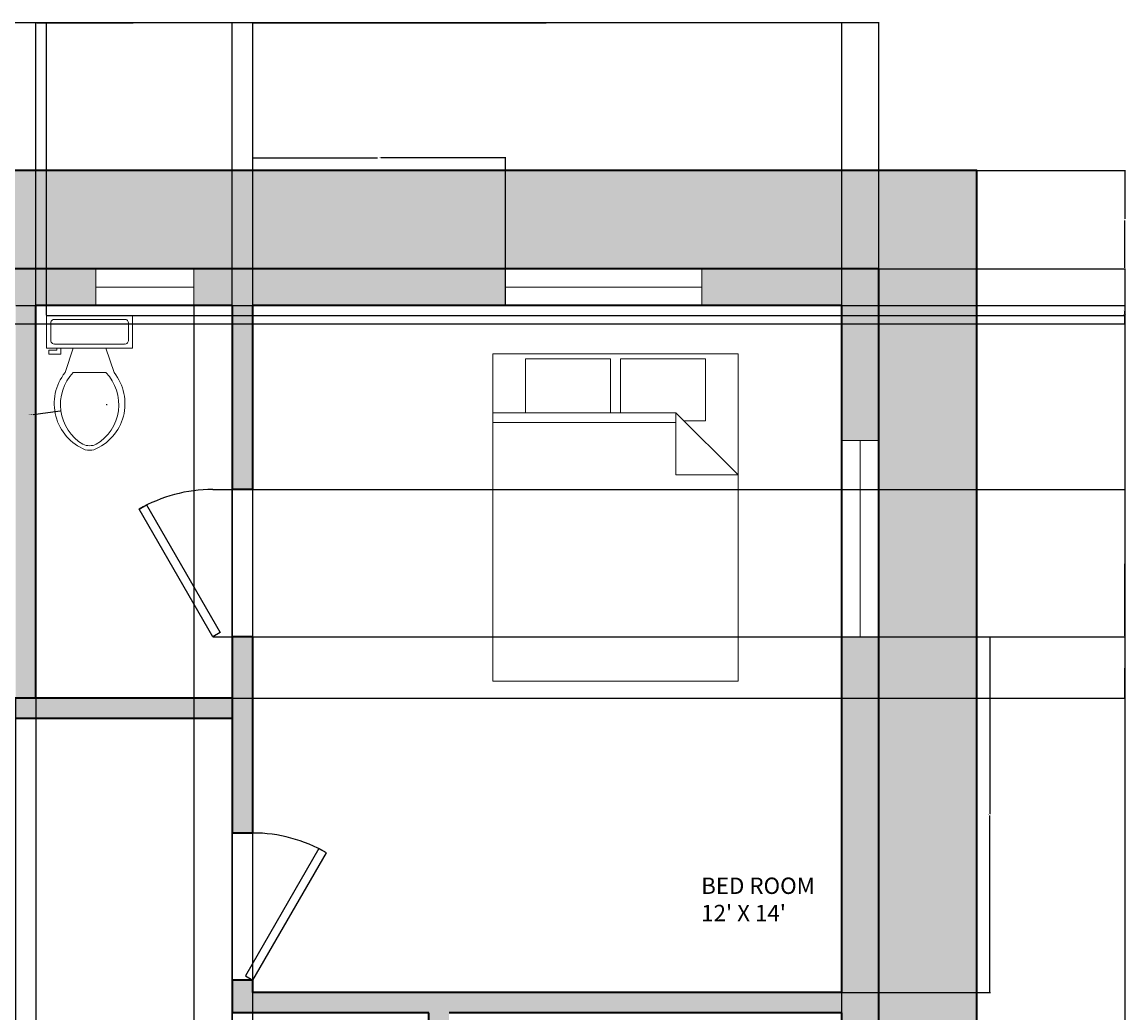
# Model space of a CAD drawing. Units: inches. Extents: x -7 to 546, y -27 to 766.
# Tile 9 of 9: x 276 to 546, y 524 to 766. Entities that reach past the tile are written whole.
import ezdxf

# ---------------------------------------------------------------- set-up
doc = ezdxf.new("R2010")
doc.units = ezdxf.units.IN
doc.header["$MEASUREMENT"] = 0
for name, color, linetype, lineweight in [('A-ANNO-DIMS', 2, 'Continuous', 18), ('A-AREA-IDEN', 7, 'Continuous', 18), ('A-FLOR-FIXT', 9, 'Continuous', 18), ('A-WALL', 7, 'Continuous', 35), ('C-PROP', 7, 'Continuous', 35), ('doors', 40, 'Continuous', 25), ('furniture', 220, 'Continuous', 18), ('window', 30, 'Continuous', 20)]:
    doc.layers.add(name, color=color, linetype=linetype, lineweight=lineweight)
doc.layers.add('A-WALL-PATT', color=251, linetype='Continuous', lineweight=13, true_color=0x636466)
doc.layers.add('L-PLNT-PATT', color=85, linetype='Continuous', lineweight=13, true_color=0x58ba48)
doc.styles.get("Standard").update_dxf_attribs({"font": 'arial.ttf'})
doc.dimstyles.get("Standard").update_dxf_attribs({"dimtxt": 0.18, "dimasz": 0.18, "dimexe": 0.18, "dimexo": 0.0625, "dimgap": 0.09, "dimtad": 0, "dimtih": 1, "dimtoh": 1, "dimdec": 4, "dimzin": 0, "dimdsep": 46, "dimtxsty": 'Standard', "dimcen": 0.09, "dimadec": 0, "dimazin": 0, "dimtfac": 1, "dimtdec": 4, "dimtofl": 0, "dimtmove": 0, "dimatfit": 3, "dimfxl": 1, "dimtolj": 1, "dimtzin": 0, "dimarcsym": 0})

# ---------------------------------------------------------------- blocks, each defined once
blk = doc.blocks.new('*U11')
for p, q in [((0, 0), (0, 100)), ((750, 0), (750, 100))]:
    blk.add_line(p, q)
blk.add_lwpolyline([(0, 0), (649.5, -375), (671.4, -337.1), (21.9, 37.9)], close=True)
blk.add_arc((0, 0), 750, 330, 0)
blk = doc.blocks.new('*U10')
for p, q in [((0, 0), (0, -100)), ((750, 0), (750, -100))]:
    blk.add_line(p, q)
blk.add_lwpolyline([(0, 0), (649.5, 375), (671.4, 337.1), (21.9, -37.9)], close=True)
blk.add_arc((0, 0), 750, 0, 30)
blk = doc.blocks.new('Bed - Queen')
for p, q in [((0, -80.00003), (0, 0)), ((0, 0), (59.99999, 0)), ((59.99999, 0), (59.99999, -80.00003)), ((7.99999, -1.2), (28.79998, -1.2)), ((7.99999, -14.4), (7.99999, -1.2)), ((28.79998, -1.2), (28.79998, -14.4)), ((31.19999, -1.2), (51.99999, -1.2)), ((31.19999, -14.4), (31.19999, -1.2)), ((51.99999, -1.2), (51.99999, -16.4)), ((0, -14.4), (44.8, -14.4)), ((59.99999, -29.6), (44.8, -14.4)), ((44.8, -14.4), (44.8, -29.6)), ((44.8, -16.8), (0, -16.8)), ((51.99999, -16.4), (46.79936, -16.4)), ((44.8, -29.6), (59.99999, -29.6)), ((59.99999, -80.00003), (0, -80.00003))]:
    blk.add_line(p, q)
blk = doc.blocks.new('Toilet - top')
for p, q in [((9.5, -6), (9.5, -2)), ((-8, -8.5), (-8, -8)), ((-7, -8), (-7, -9.5)), ((-4, -8), (-6, -14)), ((4, -8), (6, -14)), ((-10, -8.5), (-8, -8.5)), ((-10, -9.5), (-10, -8.5)), ((-7, -9.5), (-10, -9.5)), ((4, -14), (-4, -14))]:
    blk.add_line(p, q)
blk.add_lwpolyline([(10.5, -8), (10.5, 0), (-10.5, 0), (-10.5, -8)], close=True)
for points in [[(-9.5, -2), (-9.5, -6)], [(8.5, -1), (-8.5, -1)], [(-8.5, -7), (8.5, -7)]]:
    blk.add_lwpolyline(points)
for centre, radius, start, end in [((-8.62, -1.88), 0.884, 81.8699, 188.1301), ((8.62, -1.88), 0.884, 351.8699, 98.1301), ((-8.62, -6.12), 0.884, 171.8699, 278.1301), ((8.62, -6.12), 0.884, 261.8699, 8.1301), ((3.52, -21.58), 12.17, 141.4691, 247.9714), ((4.2, -21.82), 11.33, 136.3677, 238.9468), ((-3.52, -21.58), 12.17, 292.0284, 38.5307), ((-4.2, -21.82), 11.33, 301.053, 43.6321), ((0, -27.88), 4, 245.7318, 294.2682), ((0, -29), 4, 254.8605, 285.1395)]:
    blk.add_arc(centre, radius, start, end)
blk = doc.blocks.new('WIN-48IN')
for p, q in [((0, 9), (0, 0)), ((48, 9), (0, 9)), ((0, 9), (0, 4.5)), ((48, 0), (48, 9)), ((0, 4.5), (48, 4.5)), ((0, 0), (48, 0))]:
    blk.add_line(p, q)
blk = doc.blocks.new('WIN-24IN')
for p, q in [((0, 9), (0, 0)), ((24, 9), (0, 9)), ((0, 9), (0, 4.5)), ((24, 0), (24, 9)), ((0, 4.5), (24, 4.5)), ((0, 0), (24, 0))]:
    blk.add_line(p, q)
blk = doc.blocks.new('*D32')
at = {"layer": 'A-ANNO-DIMS', "color": 0, "lineweight": -2, "transparency": 16777216}
for p, q in [((53.23, 705.81), (53.23, 766.05)), ((53.41, 765.87), (268.94, 765.87)), ((485.05, 765.87), (269.52, 765.87)), ((485.23, 705.81), (485.23, 766.05))]:
    blk.add_line(p, q, dxfattribs=at)
at = {"layer": 'A-ANNO-DIMS', "color": 0, "transparency": 16777216}
for points in [[(53.41, 765.9), (53.41, 765.84), (53.23, 765.87)], [(485.05, 765.9), (485.05, 765.84), (485.23, 765.87)]]:
    blk.add_solid(points, dxfattribs=at)
at = {"layer": 'Defpoints', "color": 0, "transparency": 16777216}
for p in [(485.23, 765.87), (53.23, 705.74), (485.23, 705.74)]:
    blk.add_point(p, dxfattribs=at)
at = {"layer": 'A-ANNO-DIMS', "color": 0, "transparency": 16777216, "insert": (269.23, 765.87), "char_height": 0.18, "attachment_point": 5}
blk.add_mtext('\\A1;432', dxfattribs=at)
blk = doc.blocks.new('*D33')
at = {"layer": 'A-ANNO-DIMS', "color": 0, "lineweight": -2, "transparency": 16777216}
for p, q in [((485.29, 705.74), (545.54, 705.74)), ((545.36, 705.56), (545.36, 357.93)), ((545.36, 9.92), (545.36, 357.56)), ((461.29, 9.74), (545.54, 9.74))]:
    blk.add_line(p, q, dxfattribs=at)
at = {"layer": 'A-ANNO-DIMS', "color": 0, "transparency": 16777216}
for points in [[(545.33, 705.56), (545.39, 705.56), (545.36, 705.74)], [(545.33, 9.92), (545.39, 9.92), (545.36, 9.74)]]:
    blk.add_solid(points, dxfattribs=at)
at = {"layer": 'Defpoints', "color": 0, "transparency": 16777216}
for p in [(485.23, 705.74), (461.23, 9.74), (545.36, 9.74)]:
    blk.add_point(p, dxfattribs=at)
at = {"layer": 'A-ANNO-DIMS', "color": 0, "transparency": 16777216, "insert": (545.36, 357.74), "char_height": 0.18, "attachment_point": 5}
blk.add_mtext('\\A1;696', dxfattribs=at)
blk = doc.blocks.new('*D35')
at = {"layer": 'A-ANNO-DIMS', "color": 0, "lineweight": -2, "transparency": 16777216}
for p, q in [((509.29, 729.74), (545.54, 729.74)), ((545.36, 729.56), (545.36, 717.92)), ((545.36, 705.92), (545.36, 717.56)), ((485.29, 705.74), (545.54, 705.74))]:
    blk.add_line(p, q, dxfattribs=at)
at = {"layer": 'A-ANNO-DIMS', "color": 0, "transparency": 16777216}
for points in [[(545.33, 729.56), (545.39, 729.56), (545.36, 729.74)], [(545.33, 705.92), (545.39, 705.92), (545.36, 705.74)]]:
    blk.add_solid(points, dxfattribs=at)
at = {"layer": 'Defpoints', "color": 0, "transparency": 16777216}
for p in [(509.23, 729.74), (485.23, 705.74), (545.36, 705.74)]:
    blk.add_point(p, dxfattribs=at)
at = {"layer": 'A-ANNO-DIMS', "color": 0, "transparency": 16777216, "insert": (545.36, 717.74), "char_height": 0.18, "attachment_point": 5}
blk.add_mtext('\\A1;24', dxfattribs=at)
blk = doc.blocks.new('*D37')
at = {"layer": 'A-ANNO-DIMS', "color": 0, "lineweight": -2, "transparency": 16777216}
for p, q in [((279.23, 696.81), (279.23, 766.05)), ((279.41, 765.87), (303.01, 765.87)), ((327.05, 765.87), (303.45, 765.87)), ((327.23, 696.81), (327.23, 766.05))]:
    blk.add_line(p, q, dxfattribs=at)
at = {"layer": 'A-ANNO-DIMS', "color": 0, "transparency": 16777216}
for points in [[(279.41, 765.9), (279.41, 765.84), (279.23, 765.87)], [(327.05, 765.9), (327.05, 765.84), (327.23, 765.87)]]:
    blk.add_solid(points, dxfattribs=at)
at = {"layer": 'Defpoints', "color": 0, "transparency": 16777216}
for p in [(327.23, 765.87), (279.23, 696.74), (327.23, 696.74)]:
    blk.add_point(p, dxfattribs=at)
at = {"layer": 'A-ANNO-DIMS', "color": 0, "transparency": 16777216, "insert": (303.23, 765.87), "char_height": 0.18, "attachment_point": 5}
blk.add_mtext('\\A1;48', dxfattribs=at)
blk = doc.blocks.new('*D40')
at = {"layer": 'A-ANNO-DIMS', "color": 0, "lineweight": -2, "transparency": 16777216}
for p, q in [((327.29, 651.74), (545.54, 651.74)), ((545.36, 651.56), (545.36, 633.93)), ((545.36, 615.92), (545.36, 633.56)), ((327.29, 615.74), (545.54, 615.74))]:
    blk.add_line(p, q, dxfattribs=at)
at = {"layer": 'A-ANNO-DIMS', "color": 0, "transparency": 16777216}
for points in [[(545.33, 651.56), (545.39, 651.56), (545.36, 651.74)], [(545.33, 615.92), (545.39, 615.92), (545.36, 615.74)]]:
    blk.add_solid(points, dxfattribs=at)
at = {"layer": 'Defpoints', "color": 0, "transparency": 16777216}
for p in [(327.23, 651.74), (545.36, 651.74), (327.23, 615.74)]:
    blk.add_point(p, dxfattribs=at)
at = {"layer": 'A-ANNO-DIMS', "color": 0, "transparency": 16777216, "insert": (545.36, 633.74), "char_height": 0.18, "attachment_point": 5}
blk.add_mtext('\\A1;36', dxfattribs=at)
blk = doc.blocks.new('*D41')
at = {"layer": 'A-ANNO-DIMS', "color": 0, "lineweight": -2, "transparency": 16777216}
for p, q in [((274.23, 600.68), (274.23, -26.56)), ((279.23, 600.68), (279.23, -26.56)), ((274.41, -26.38), (276.58, -26.38)), ((279.05, -26.38), (276.88, -26.38))]:
    blk.add_line(p, q, dxfattribs=at)
at = {"layer": 'A-ANNO-DIMS', "color": 0, "transparency": 16777216}
for points in [[(274.41, -26.35), (274.41, -26.41), (274.23, -26.38)], [(279.05, -26.35), (279.05, -26.41), (279.23, -26.38)]]:
    blk.add_solid(points, dxfattribs=at)
at = {"layer": 'Defpoints', "color": 0, "transparency": 16777216}
for p in [(274.23, 600.74), (279.23, 600.74), (279.23, -26.38)]:
    blk.add_point(p, dxfattribs=at)
at = {"layer": 'A-ANNO-DIMS', "color": 0, "transparency": 16777216, "insert": (276.73, -26.38), "char_height": 0.18, "attachment_point": 5}
blk.add_mtext('\\A1;5', dxfattribs=at)
blk = doc.blocks.new('*D43')
at = {"layer": 'A-ANNO-DIMS', "color": 0, "lineweight": -2, "transparency": 16777216}
for p, q in [((317.84, 696.68), (317.84, -26.56)), ((327.23, 696.68), (327.23, -26.56)), ((318.02, -26.38), (322.21, -26.38)), ((327.05, -26.38), (322.86, -26.38))]:
    blk.add_line(p, q, dxfattribs=at)
at = {"layer": 'A-ANNO-DIMS', "color": 0, "transparency": 16777216}
for points in [[(318.02, -26.35), (318.02, -26.41), (317.84, -26.38)], [(327.05, -26.35), (327.05, -26.41), (327.23, -26.38)]]:
    blk.add_solid(points, dxfattribs=at)
at = {"layer": 'Defpoints', "color": 0, "transparency": 16777216}
for p in [(317.84, 696.74), (327.23, 696.74), (327.23, -26.38)]:
    blk.add_point(p, dxfattribs=at)
at = {"layer": 'A-ANNO-DIMS', "color": 0, "transparency": 16777216, "insert": (322.54, -26.38), "char_height": 0.18, "attachment_point": 5}
blk.add_mtext('\\A1;9.39', dxfattribs=at)
blk = doc.blocks.new('*D44')
at = {"layer": 'A-ANNO-DIMS', "color": 0, "lineweight": -2, "transparency": 16777216}
for p, q in [((327.29, 615.74), (545.54, 615.74)), ((545.36, 615.56), (545.36, 608.43)), ((545.36, 600.92), (545.36, 608.06)), ((327.29, 600.74), (545.54, 600.74))]:
    blk.add_line(p, q, dxfattribs=at)
at = {"layer": 'A-ANNO-DIMS', "color": 0, "transparency": 16777216}
for points in [[(545.33, 615.56), (545.39, 615.56), (545.36, 615.74)], [(545.33, 600.92), (545.39, 600.92), (545.36, 600.74)]]:
    blk.add_solid(points, dxfattribs=at)
at = {"layer": 'Defpoints', "color": 0, "transparency": 16777216}
for p in [(327.23, 615.74), (545.36, 615.74), (327.23, 600.74)]:
    blk.add_point(p, dxfattribs=at)
at = {"layer": 'A-ANNO-DIMS', "color": 0, "transparency": 16777216, "insert": (545.36, 608.24), "char_height": 0.18, "attachment_point": 5}
blk.add_mtext('\\A1;15', dxfattribs=at)
blk = doc.blocks.new('*D57')
at = {"layer": 'A-ANNO-DIMS', "color": 0, "lineweight": -2, "transparency": 16777216}
for p, q in [((332.23, 273.81), (332.23, 766.05)), ((332.41, 765.87), (403.95, 765.87)), ((476.05, 765.87), (404.51, 765.87)), ((476.23, 273.81), (476.23, 766.05))]:
    blk.add_line(p, q, dxfattribs=at)
at = {"layer": 'A-ANNO-DIMS', "color": 0, "transparency": 16777216}
for points in [[(332.41, 765.9), (332.41, 765.84), (332.23, 765.87)], [(476.05, 765.9), (476.05, 765.84), (476.23, 765.87)]]:
    blk.add_solid(points, dxfattribs=at)
at = {"layer": 'Defpoints', "color": 0, "transparency": 16777216}
for p in [(476.23, 765.87), (332.23, 273.74), (476.23, 273.74)]:
    blk.add_point(p, dxfattribs=at)
at = {"layer": 'A-ANNO-DIMS', "color": 0, "transparency": 16777216, "insert": (404.23, 765.87), "char_height": 0.18, "attachment_point": 5}
blk.add_mtext('\\A1;144', dxfattribs=at)
blk = doc.blocks.new('*D70')
at = {"layer": 'A-ANNO-DIMS', "color": 0, "lineweight": -2, "transparency": 16777216}
for p, q in [((332.23, 696.81), (332.23, 733.05)), ((332.41, 732.87), (362.71, 732.87)), ((393.79, 732.87), (363.5, 732.87)), ((393.97, 696.81), (393.97, 733.05))]:
    blk.add_line(p, q, dxfattribs=at)
at = {"layer": 'A-ANNO-DIMS', "color": 0, "transparency": 16777216}
for points in [[(332.41, 732.9), (332.41, 732.84), (332.23, 732.87)], [(393.79, 732.9), (393.79, 732.84), (393.97, 732.87)]]:
    blk.add_solid(points, dxfattribs=at)
at = {"layer": 'Defpoints', "color": 0, "transparency": 16777216}
for p in [(393.97, 732.87), (332.23, 696.74), (393.97, 696.74)]:
    blk.add_point(p, dxfattribs=at)
at = {"layer": 'A-ANNO-DIMS', "color": 0, "transparency": 16777216, "insert": (363.1, 732.87), "char_height": 0.18, "attachment_point": 5}
blk.add_mtext('\\A1;61.74', dxfattribs=at)
blk = doc.blocks.new('*D75')
at = {"layer": 'A-ANNO-DIMS', "color": 0, "lineweight": -2, "transparency": 16777216}
for p, q in [((476.29, 615.69), (512.54, 615.69)), ((512.36, 615.51), (512.36, 572.4)), ((512.36, 528.92), (512.36, 572.03)), ((476.29, 528.74), (512.54, 528.74))]:
    blk.add_line(p, q, dxfattribs=at)
at = {"layer": 'A-ANNO-DIMS', "color": 0, "transparency": 16777216}
for points in [[(512.33, 615.51), (512.39, 615.51), (512.36, 615.69)], [(512.33, 528.92), (512.39, 528.92), (512.36, 528.74)]]:
    blk.add_solid(points, dxfattribs=at)
at = {"layer": 'Defpoints', "color": 0, "transparency": 16777216}
for p in [(476.23, 615.69), (476.23, 528.74), (512.36, 528.74)]:
    blk.add_point(p, dxfattribs=at)
at = {"layer": 'A-ANNO-DIMS', "color": 0, "transparency": 16777216, "insert": (512.36, 572.22), "char_height": 0.18, "attachment_point": 5}
blk.add_mtext('\\A1;86.95', dxfattribs=at)
blk = doc.blocks.new('*D81')
at = {"layer": 'A-ANNO-DIMS', "color": 0, "lineweight": -2, "transparency": 16777216}
for p, q in [((62.23, 240.81), (62.23, 766.05)), ((62.41, 765.87), (194.44, 765.87)), ((327.05, 765.87), (195.02, 765.87)), ((327.23, 234.81), (327.23, 766.05))]:
    blk.add_line(p, q, dxfattribs=at)
at = {"layer": 'A-ANNO-DIMS', "color": 0, "transparency": 16777216}
for points in [[(62.41, 765.9), (62.41, 765.84), (62.23, 765.87)], [(327.05, 765.9), (327.05, 765.84), (327.23, 765.87)]]:
    blk.add_solid(points, dxfattribs=at)
at = {"layer": 'Defpoints', "color": 0, "transparency": 16777216}
for p in [(327.23, 765.87), (62.23, 240.74), (327.23, 234.74)]:
    blk.add_point(p, dxfattribs=at)
at = {"layer": 'A-ANNO-DIMS', "color": 0, "transparency": 16777216, "insert": (194.73, 765.87), "char_height": 0.18, "attachment_point": 5}
blk.add_mtext('\\A1;265', dxfattribs=at)
blk = doc.blocks.new('*D86')
at = {"layer": 'A-ANNO-DIMS', "color": 0, "lineweight": -2, "transparency": 16777216}
for p, q in [((274.29, 696.74), (545.54, 696.74)), ((545.36, 696.56), (545.36, 694.67)), ((545.36, 692.41), (545.36, 694.31)), ((268.8, 692.23), (545.54, 692.23))]:
    blk.add_line(p, q, dxfattribs=at)
at = {"layer": 'A-ANNO-DIMS', "color": 0, "transparency": 16777216}
for points in [[(545.33, 696.56), (545.39, 696.56), (545.36, 696.74)], [(545.33, 692.41), (545.39, 692.41), (545.36, 692.23)]]:
    blk.add_solid(points, dxfattribs=at)
at = {"layer": 'Defpoints', "color": 0, "transparency": 16777216}
for p in [(274.23, 696.74), (268.74, 692.23), (545.36, 692.23)]:
    blk.add_point(p, dxfattribs=at)
at = {"layer": 'A-ANNO-DIMS', "color": 0, "transparency": 16777216, "insert": (545.36, 694.49), "char_height": 0.18, "attachment_point": 5}
blk.add_mtext('\\A1;4.512', dxfattribs=at)
blk = doc.blocks.new('*D87')
at = {"layer": 'A-ANNO-DIMS', "color": 0, "lineweight": -2, "transparency": 16777216}
for p, q in [((279.23, 696.81), (279.23, 766.05)), ((279.41, 765.87), (280.14, 765.87)), ((281.66, 765.87), (280.93, 765.87)), ((281.84, 694.39), (281.84, 766.05))]:
    blk.add_line(p, q, dxfattribs=at)
at = {"layer": 'A-ANNO-DIMS', "color": 0, "transparency": 16777216}
for points in [[(279.41, 765.9), (279.41, 765.84), (279.23, 765.87)], [(281.66, 765.9), (281.66, 765.84), (281.84, 765.87)]]:
    blk.add_solid(points, dxfattribs=at)
at = {"layer": 'Defpoints', "color": 0, "transparency": 16777216}
for p in [(281.84, 765.87), (279.23, 696.74), (281.84, 694.32)]:
    blk.add_point(p, dxfattribs=at)
at = {"layer": 'A-ANNO-DIMS', "color": 0, "transparency": 16777216, "insert": (280.54, 765.87), "char_height": 0.18, "attachment_point": 5}
blk.add_mtext('\\A1;2.608', dxfattribs=at)
blk = doc.blocks.new('*D88')
at = {"layer": 'A-ANNO-DIMS', "color": 0, "lineweight": -2, "transparency": 16777216}
for p, q in [((279.29, 696.74), (545.54, 696.74)), ((545.36, 696.56), (545.36, 695.71)), ((281.9, 694.32), (545.54, 694.32)), ((545.36, 694.5), (545.36, 695.35))]:
    blk.add_line(p, q, dxfattribs=at)
at = {"layer": 'A-ANNO-DIMS', "color": 0, "transparency": 16777216}
for points in [[(545.33, 696.56), (545.39, 696.56), (545.36, 696.74)], [(545.33, 694.5), (545.39, 694.5), (545.36, 694.32)]]:
    blk.add_solid(points, dxfattribs=at)
at = {"layer": 'Defpoints', "color": 0, "transparency": 16777216}
for p in [(279.23, 696.74), (281.84, 694.32), (545.36, 694.32)]:
    blk.add_point(p, dxfattribs=at)
at = {"layer": 'A-ANNO-DIMS', "color": 0, "transparency": 16777216, "insert": (545.36, 695.53), "char_height": 0.18, "attachment_point": 5}
blk.add_mtext('\\A1;2.42', dxfattribs=at)
blk = doc.blocks.new('*D94')
at = {"layer": 'A-ANNO-DIMS', "color": 0, "lineweight": -2, "transparency": 16777216}
for p, q in [((296.45, 672.51), (296.63, 672.51)), ((296.54, 672.42), (296.54, 672.6)), ((278.57, 670.09), (285.13, 670.97))]:
    blk.add_line(p, q, dxfattribs=at)
at = {"layer": 'A-ANNO-DIMS', "color": 0, "transparency": 16777216}
blk.add_solid([(285.13, 671), (285.14, 670.94), (285.31, 671)], dxfattribs=at)
at = {"layer": 'Defpoints', "color": 0, "transparency": 16777216}
for p in [(296.54, 672.51), (285.31, 671)]:
    blk.add_point(p, dxfattribs=at)
at = {"layer": 'A-ANNO-DIMS', "color": 0, "transparency": 16777216, "insert": (277.9, 670.09), "char_height": 0.18, "attachment_point": 5}
blk.add_mtext('\\A1;6X R11.33', dxfattribs=at)

msp = doc.modelspace()

# ---------------------------------------------------------------- hatches: boundary and pattern name
at = {"layer": 'A-WALL-PATT'}
h = msp.add_hatch(color=256, dxfattribs=at)
h.dxf.hatch_style = 1
h.paths.add_polyline_path([(62.2319, 696.744), (86.6896, 696.744), (86.6896, 705.744), (53.2319, 705.744), (53.2319, 627.8642), (57.7271, 627.8642), (62.2319, 627.8642)])
h.paths.add_polyline_path([(229.7414, 705.744), (134.6896, 705.744), (134.6896, 696.744), (206.2319, 696.744), (206.2319, 567.744), (211.2319, 567.744), (211.2319, 595.744), (214.2319, 595.744), (214.2319, 600.744), (211.2319, 600.744), (211.2319, 696.744), (229.7414, 696.744)])
h.paths.add_polyline_path([(293.8423, 705.744), (253.7414, 705.744), (253.7414, 696.744), (274.2319, 696.744), (274.2319, 600.744), (279.2319, 600.744), (279.2319, 696.744), (293.8423, 696.744)])
h.paths.add_polyline_path([(393.9743, 705.744), (317.8423, 705.744), (317.8423, 696.744), (327.2319, 696.744), (327.2319, 651.744), (332.2319, 651.744), (332.2319, 696.744), (393.9743, 696.744)])
h.paths.add_polyline_path([(485.2319, 705.744), (441.9743, 705.744), (441.9743, 696.744), (476.2319, 696.744), (476.2319, 663.6898), (480.7319, 663.6898), (485.2319, 663.6898)])
h.paths.add_polyline_path([(485.2319, 615.6898), (476.2319, 615.6898), (476.2319, 528.744), (332.2319, 528.744), (332.2319, 531.744), (327.2319, 531.744), (327.2319, 523.744), (375.2319, 523.744), (375.2319, 427.744), (327.2319, 427.744), (327.2319, 419.744), (332.2319, 419.744), (332.2319, 422.744), (413.089, 422.744), (413.089, 427.744), (380.2319, 427.744), (380.2319, 523.744), (476.2319, 523.744), (476.2319, 490.9334), (485.2319, 490.9334)])
h.paths.add_polyline_path([(485.2319, 466.9334), (476.2319, 466.9334), (476.2319, 370.0932), (480.7319, 370.0932), (485.2319, 370.0932)])
h.paths.add_polyline_path([(485.2319, 322.0932), (476.2319, 322.0932), (476.2319, 278.744), (332.2319, 278.744), (332.2319, 383.744), (327.2319, 383.744), (327.2319, 273.744), (327.2319, 270.744), (332.2319, 270.744), (332.2319, 273.744), (476.2319, 273.744), (476.2319, 201.0338), (480.7319, 201.0338), (485.2319, 201.0338)])
h.paths.add_polyline_path([(485.2319, 153.0338), (476.2319, 153.0338), (476.2319, 42.744), (461.2319, 42.744), (461.2319, 33.744), (485.2319, 33.744)])
h.paths.add_polyline_path([(332.2319, 234.744), (327.2319, 234.744), (327.2319, 160.744), (315.2319, 160.744), (315.2319, 151.744), (327.2319, 151.744), (327.2319, 33.744), (332.2319, 33.744)])
h.paths.add_polyline_path([(252.2319, 151.744), (258.4464, 151.744), (264.2319, 151.744), (264.2319, 160.744), (252.2319, 160.744), (252.2319, 172.744), (247.2319, 172.744), (247.2319, 91.744), (127.2319, 91.744), (127.2319, 196.744), (122.2319, 196.744), (122.2319, 91.744), (62.2319, 91.744), (62.2319, 126.1124), (53.2319, 126.1124), (53.2319, 9.744), (62.2319, 9.744), (62.2319, 86.744), (247.2319, 86.744), (247.2319, 33.744), (252.2319, 33.744), (252.2319, 53.744)])
h.paths.add_polyline_path([(62.2319, 235.744), (122.2319, 235.744), (122.2319, 232.744), (127.2319, 232.744), (127.2319, 235.744), (247.2319, 235.744), (247.2319, 220.744), (252.2319, 220.744), (252.2319, 240.744), (250.6678, 240.744), (247.2319, 240.744), (62.2319, 240.744), (62.2319, 322.0932), (53.2319, 322.0932), (53.2319, 174.1124), (57.7271, 174.1124), (62.2319, 174.1124)])
h = msp.add_hatch(color=256, dxfattribs=at)
h.dxf.hatch_style = 1
h.paths.add_polyline_path([(327.2319, 600.744), (252.2319, 600.744), (252.2319, 595.744), (327.2319, 595.744)])
h.paths.add_polyline_path([(332.2319, 615.744), (327.2319, 615.744), (327.2319, 567.744), (332.2319, 567.744)])
h.paths.add_polyline_path([(252.2319, 600.744), (250.2319, 600.744), (250.2319, 595.744), (252.2319, 595.744)])
at = {"layer": 'L-PLNT-PATT'}
h = msp.add_hatch(color=256, dxfattribs=at)
h.dxf.hatch_style = 1
h.paths.add_polyline_path([(509.2319, 729.744), (29.2319, 729.744), (29.2319, 9.744), (53.2319, 9.744), (53.2319, 705.744), (485.2319, 705.744), (485.2319, 33.744), (461.2319, 33.744), (461.2319, 9.744), (509.2319, 9.744)])

# ---------------------------------------------------------------- linework, layer by layer
at = {"layer": 'A-WALL'}
for p, q in [((279.2319, 600.744), (279.2319, 696.744)), ((327.2319, 696.744), (279.2319, 696.744)), ((327.2319, 651.744), (327.2319, 696.744)), ((327.2319, 651.744), (327.2319, 696.744)), ((332.2319, 651.744), (332.2319, 696.744)), ((332.2319, 651.744), (332.2319, 696.744)), ((476.2319, 696.744), (332.2319, 696.744)), ((476.2319, 528.744), (476.2319, 696.744)), ((332.2319, 651.744), (327.2319, 651.744)), ((327.2319, 567.744), (327.2319, 615.744)), ((327.2319, 600.744), (327.2319, 615.744)), ((332.2319, 615.744), (327.2319, 615.744)), ((332.2319, 567.744), (332.2319, 615.744)), ((332.2319, 567.744), (332.2319, 615.744)), ((332.2319, 600.744), (332.2319, 615.744)), ((327.2319, 600.744), (250.2319, 600.744)), ((327.2319, 595.744), (250.2319, 595.744)), ((327.2319, 567.744), (327.2319, 595.744)), ((332.2319, 567.744), (327.2319, 567.744)), ((327.2319, 523.744), (327.2319, 531.744)), ((327.2319, 523.744), (327.2319, 531.744)), ((332.2319, 531.744), (327.2319, 531.744)), ((332.2319, 528.744), (332.2319, 531.744)), ((332.2319, 528.744), (332.2319, 531.744)), ((476.2319, 528.744), (332.2319, 528.744)), ((375.2319, 523.744), (327.2319, 523.744)), ((375.2319, 427.744), (375.2319, 523.744)), ((476.2319, 523.744), (380.2319, 523.744)), ((476.2319, 278.744), (476.2319, 523.744))]:
    msp.add_line(p, q, dxfattribs=at)
msp.add_lwpolyline([(461.2319, 33.744), (485.2319, 33.744), (485.2319, 705.744), (53.2319, 705.744), (53.2319, 9.744)], dxfattribs=at)
at = {"layer": 'C-PROP'}
msp.add_lwpolyline([(29.2319, 9.744), (509.2319, 9.744), (509.2319, 729.744), (29.2319, 729.744)], close=True, dxfattribs=at)

# ---------------------------------------------------------------- block references
at = {"layer": 'A-FLOR-FIXT'}
msp.add_blockref('Toilet - top', (292.3398, 694.3236), dxfattribs=at)
at = {"layer": 'doors', "xscale": 0.0480000000000013, "yscale": 0.0480000000000013, "zscale": 0.0480000000000013, "rotation": 90}
for name, p in [('*U10', (322.4319, 615.744)), ('*U11', (332.2319, 531.744))]:
    msp.add_blockref(name, p, dxfattribs=at)
at = {"layer": 'furniture'}
msp.add_blockref('Bed - Queen', (390.8772, 684.899), dxfattribs=at)
at = {"layer": 'window'}
for name, p in [('WIN-24IN', (293.8418, 696.744)), ('WIN-48IN', (393.9747, 696.744))]:
    msp.add_blockref(name, p, dxfattribs=at)
at = {"layer": 'window', "extrusion": (0, 0, -1), "zscale": -1, "rotation": 270.0000000000001}
msp.add_blockref('WIN-48IN', (-485.2319, 663.6894), dxfattribs=at)

# ---------------------------------------------------------------- texts
at = {"layer": 'A-AREA-IDEN', "insert": (441.8428, 556.8412), "char_height": 4, "attachment_point": 1}
msp.add_mtext_dynamic_manual_height_columns("BED ROOM\\P12' X 14'", width=80.777321, gutter_width=1, heights=[0], dxfattribs=at)

# ---------------------------------------------------------------- dimensions: what is measured, and where the dimension line sits
at = {"layer": 'A-ANNO-DIMS'}
for base, p1, p2, override, picture, middle in [((485.2319, 765.869), (53.2319, 705.744), (485.2319, 705.744), {"dimdec": 0, "dimlfac": 1, "dimrnd": 0, "dimzin": 0, "dimdsep": 46, "dimlunit": 2}, '*D32', (269.2319, 765.869)), ((327.2319, 765.869), (62.2319, 240.744), (327.2319, 234.744), {"dimdec": 0, "dimlfac": 1, "dimrnd": 0, "dimzin": 0, "dimdsep": 46, "dimlunit": 2}, '*D81', (194.7319, 765.869)), ((327.2319, 765.869), (279.2319, 696.744), (327.2319, 696.744), {"dimdec": 0, "dimlfac": 1, "dimrnd": 0, "dimzin": 0, "dimdsep": 46, "dimlunit": 2}, '*D37', (303.2319, 765.869)), ((281.8398, 765.869), (279.2319, 696.744), (281.8398, 694.3236), {"dimdec": 3, "dimlfac": 1, "dimrnd": 0, "dimzin": 0, "dimdsep": 46, "dimlunit": 2}, '*D87', (280.5358, 765.869)), ((476.2319, 765.869), (332.2319, 273.744), (476.2319, 273.744), {"dimdec": 0, "dimlfac": 1, "dimrnd": 0, "dimzin": 0, "dimdsep": 46, "dimlunit": 2}, '*D57', (404.2319, 765.869)), ((393.9743, 732.869), (332.2319, 696.744), (393.9743, 696.744), {"dimdec": 2, "dimlfac": 1, "dimrnd": 0, "dimzin": 0, "dimdsep": 46, "dimlunit": 2}, '*D70', (363.1031, 732.869)), ((327.2319, -26.381), (317.8423, 696.744), (327.2319, 696.744), {"dimdec": 2, "dimlfac": 1, "dimrnd": 0, "dimzin": 0, "dimdsep": 46, "dimlunit": 2}, '*D43', (322.5371, -26.381)), ((279.2319, -26.381), (274.2319, 600.744), (279.2319, 600.744), {"dimdec": 0, "dimlfac": 1, "dimrnd": 0, "dimzin": 0, "dimdsep": 46, "dimlunit": 2}, '*D41', (276.7319, -26.381))]:
    dim = msp.add_linear_dim(base=base, p1=p1, p2=p2, dimstyle='Standard', override=override, dxfattribs=at)
    dim.commit()
    dim.dimension.update_dxf_attribs({"geometry": picture, "text_midpoint": middle})
for base, p1, p2, angle, override, picture, middle in [((545.3569, 705.744), (509.2319, 729.744), (485.2319, 705.744), 90, {"dimdec": 0, "dimlfac": 1, "dimrnd": 0, "dimzin": 0, "dimdsep": 46, "dimlunit": 2}, '*D35', (545.3569, 717.744)), ((545.3569, 9.744), (485.2319, 705.744), (461.2319, 9.744), 90, {"dimdec": 0, "dimlfac": 1, "dimrnd": 0, "dimzin": 0, "dimdsep": 46, "dimlunit": 2}, '*D33', (545.3569, 357.744)), ((545.3569, 692.2322), (274.2319, 696.744), (268.7385, 692.2322), 90, {"dimdec": 3, "dimlfac": 1, "dimrnd": 0, "dimzin": 0, "dimdsep": 46, "dimlunit": 2}, '*D86', (545.3569, 694.4881)), ((545.3569, 694.3236), (279.2319, 696.744), (281.8398, 694.3236), 90, {"dimdec": 2, "dimlfac": 1, "dimrnd": 0, "dimzin": 0, "dimdsep": 46, "dimlunit": 2}, '*D88', (545.3569, 695.5338)), ((545.3569, 651.744), (327.2319, 615.744), (327.2319, 651.744), 90, {"dimdec": 0, "dimlfac": 1, "dimrnd": 0, "dimzin": 0, "dimdsep": 46, "dimlunit": 2}, '*D40', (545.3569, 633.744)), ((545.3569, 615.744), (327.2319, 600.744), (327.2319, 615.744), 90, {"dimdec": 0, "dimlfac": 1, "dimrnd": 0, "dimzin": 0, "dimdsep": 46, "dimlunit": 2}, '*D44', (545.3569, 608.244)), ((512.3569, 528.744), (476.2319, 615.6898), (476.2319, 528.744), 270, {"dimdec": 2, "dimlfac": 1, "dimrnd": 0, "dimzin": 0, "dimdsep": 46, "dimlunit": 2}, '*D75', (512.3569, 572.2169))]:
    dim = msp.add_linear_dim(base=base, p1=p1, p2=p2, angle=angle, dimstyle='Standard', override=override, dxfattribs=at)
    dim.commit()
    dim.dimension.update_dxf_attribs({"geometry": picture, "text_midpoint": middle})
dim = msp.add_radius_dim(center=(296.5397, 672.5062), mpoint=(285.3115, 670.9969), text='6X <>', dimstyle='Standard', override={"dimdec": 2, "dimlfac": 1, "dimrnd": 0, "dimzin": 0, "dimdsep": 46, "dimlunit": 2}, dxfattribs=at)
dim.commit()
dim.dimension.update_dxf_attribs({"geometry": '*D94', "text_midpoint": (278.5746, 670.0914), "dimtype": 164})

doc.saveas('drawing.dxf')
